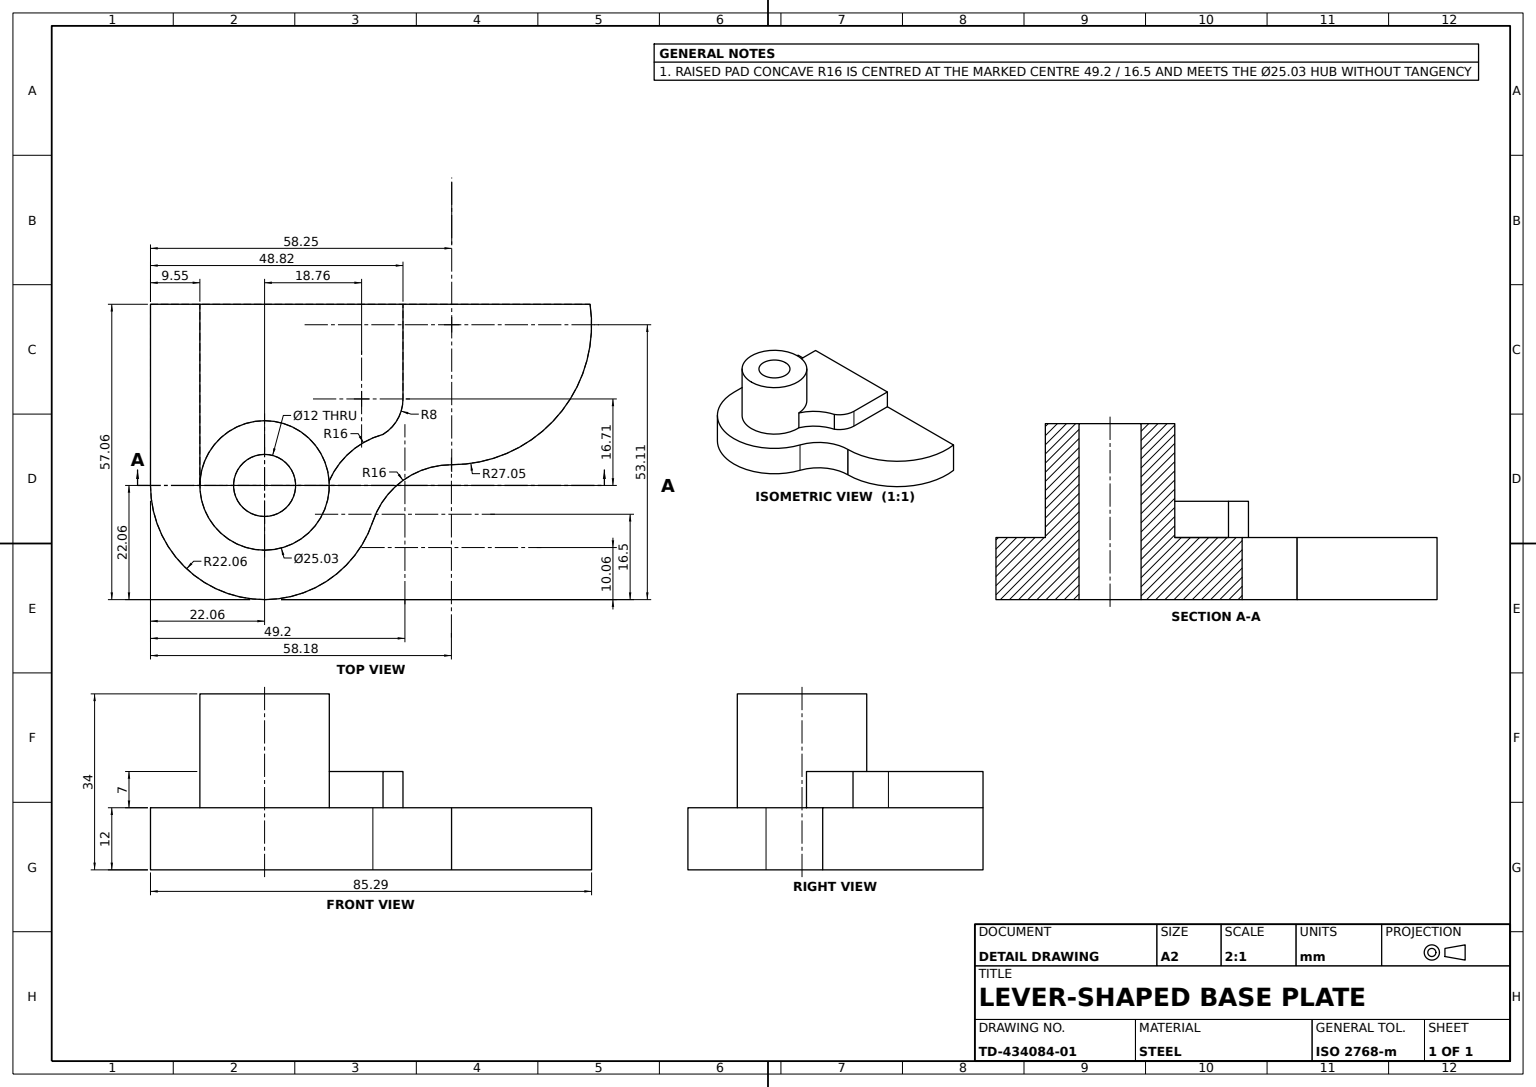
from build123d import *

# Parameters (mm, degrees)
BASE_PLATE_DEPTH   = 12
RAISED_PAD_DEPTH   = 7
HUB_BOSS_PROFILE_R = 12.512998998
HUB_BOSS_DEPTH     = 15
BORE_12_PROFILE_R  = 6
BORE_12_DEPTH      = 68


with BuildPart() as part:
    # Base Plate Profile → Base Plate (new body)
    with BuildSketch(Plane(origin=(0, 0, 0), x_dir=(1, 0, 0), z_dir=(0, 1, 0))):
        with BuildLine():
            Line((-22.062998998, 0), (-22.062998998, 35))
            Line((-22.062998998, 35), (62.937001002, 35))
            ThreePointArc((62.937001002, 35), (56.656926651, 13.374824859), (36.182547719, 4))
            Line((36.182547719, 4), (36.121903227, 4))
            ThreePointArc((36.121903227, 4), (26.759967036, 0.975135867), (20.93785397, -6.955731155))
            ThreePointArc((20.93785397, -6.955731155), (-3.52307207, -21.779896418), (-22.062998998, 0))
        make_face()
    extrude(amount=BASE_PLATE_DEPTH)

    # Raised Pad Profile → Raised Pad (add)
    with BuildSketch(Plane(origin=(0, 12, 0), x_dir=(1, 0, 0), z_dir=(0, 1, 0))):
        with BuildLine():
            Line((-12.512998998, 35), (-12.512998998, 0))
            ThreePointArc((-12.512998998, 0), (0.432197973, -12.505532729), (12.483142832, 0.863880178))
            ThreePointArc((12.483142832, 0.863880178), (16.674295928, 6.54084856), (22.899922014, 9.862792887))
            ThreePointArc((22.899922014, 9.862792887), (25.728454671, 12.778886311), (26.759967036, 16.708285768))
            Line((26.759967036, 16.708285768), (26.759967036, 35))
            Line((26.759967036, 35), (-12.512998998, 35))
        make_face()
    extrude(amount=RAISED_PAD_DEPTH)

    # Hub Boss Profile → Hub Boss (add)
    with BuildSketch(Plane(origin=(0, 19, 0), x_dir=(1, 0, 0), z_dir=(0, 1, 0))):
        with Locations(Location((0, 0, 0), (0, 0, 3.958770586))):
            Circle(HUB_BOSS_PROFILE_R)
    extrude(amount=HUB_BOSS_DEPTH)

    # Bore Ø12 Profile → Bore Ø12 (cut)
    with BuildSketch(Plane(origin=(0, 34, 0), x_dir=(1, 0, 0), z_dir=(0, 1, 0))):
        with Locations(Location((0, 0, 0), (0, 0, 270))):
            Circle(BORE_12_PROFILE_R)
    extrude(amount=-BORE_12_DEPTH, mode=Mode.SUBTRACT)


solid = part.part
